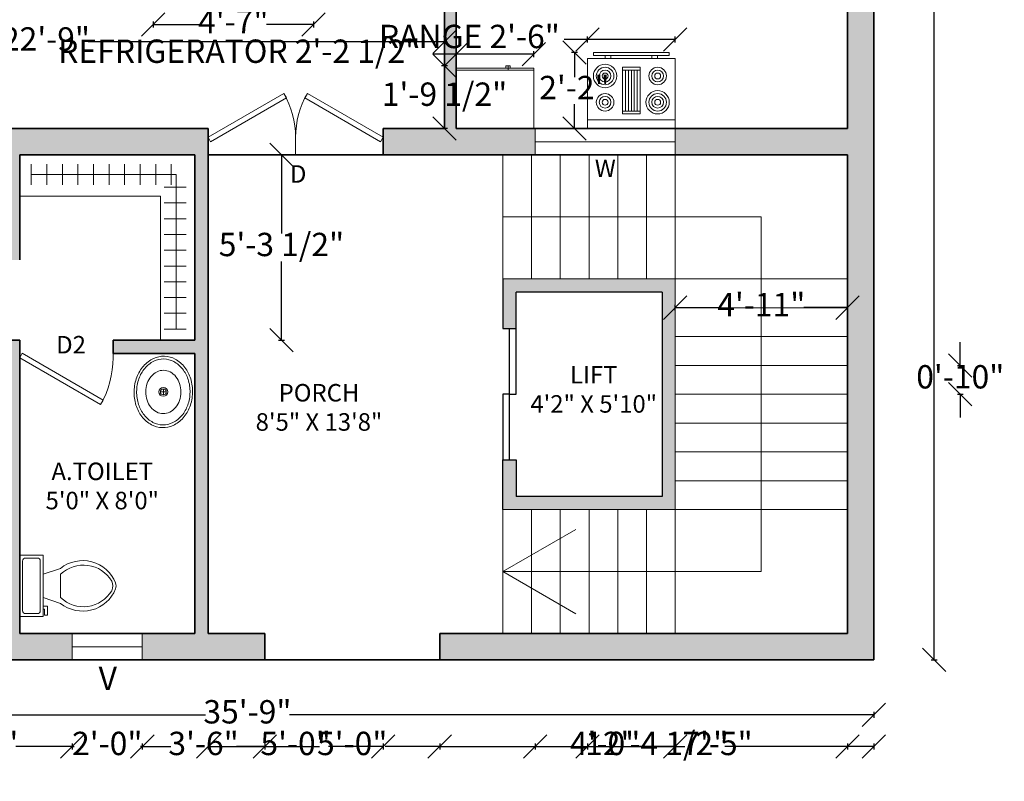
# Model space of a CAD drawing. Units: inches. Extents: x 2530 to 3100, y 543 to 1175.
# Tile 2 of 5: x 2762 to 3100, y 543 to 804. Entities that reach past the tile are written whole.
import ezdxf

# ---------------------------------------------------------------- set-up
doc = ezdxf.new("R2010")
doc.units = ezdxf.units.IN
for name, color, linetype, lineweight in [('A-ANNO-DIMS', 2, 'Continuous', 18), ('A-ANNO-TEXT', 7, 'Continuous', 18), ('A-AREA-IDEN', 7, 'Continuous', 18), ('A-DOOR', 3, 'Continuous', 18), ('A-EQPM', 8, 'Continuous', 18), ('A-FLOR-CASE', 172, 'Continuous', 13), ('A-FLOR-EVTR', 7, 'Continuous', 25), ('A-FLOR-FIXT', 8, 'Continuous', 18), ('A-FLOR-STRS', 7, 'Continuous', 18), ('A-GLAZ', 4, 'Continuous', 18), ('A-WALL', 7, 'Continuous', 35), ('A-WALL-PATT', 30, 'Continuous', 13)]:
    doc.layers.add(name, color=color, linetype=linetype, lineweight=lineweight)
doc.styles.get("Standard").update_dxf_attribs({"font": 'arial.ttf'})
doc.dimstyles.new('ISO-25', dxfattribs={"dimtxt": 8, "dimasz": 8, "dimexe": 1, "dimexo": 1, "dimtad": 0, "dimtih": 1, "dimtoh": 1, "dimlunit": 3, "dimtxsty": 'Standard', "dimblk": 'OBLIQUE', "dimcen": 2.5, "dimadec": 0, "dimazin": 0, "dimtfac": 1, "dimtmove": 0, "dimatfit": 3, "dimfxl": 1, "dimfxlon": 1, "dimarcsym": 0})

# ---------------------------------------------------------------- blocks, each defined once
blk = doc.blocks.new('*U10')
for p, q in [((0, 0), (0, 6)), ((32, 0), (32, 6))]:
    blk.add_line(p, q)
blk.add_lwpolyline([(0, 0), (27.71, -16), (28.59, -14.48), (0.87, 1.52)], close=True)
blk.add_arc((0, 0), 32, 330, 0)
blk = doc.blocks.new('*U9')
for p, q in [((0, 0), (0, -6)), ((30, 0), (30, -6))]:
    blk.add_line(p, q)
blk.add_lwpolyline([(0, 0), (25.98, 15), (26.86, 13.48), (0.87, -1.52)], close=True)
blk.add_arc((0, 0), 30, 0, 30)
blk = doc.blocks.new('*U8')
for p, q in [((-30, 0), (-30, -6)), ((0, 0), (0, -6))]:
    blk.add_line(p, q)
blk.add_lwpolyline([(0, 0), (-25.98, 15), (-26.86, 13.48), (-0.88, -1.52)], close=True)
blk.add_arc((0, 0), 30, 150, 180)
blk = doc.blocks.new('_Oblique')
at = {"color": 0, "linetype": 'ByBlock', "lineweight": -2}
blk.add_line((-0.5, -0.5), (0.5, 0.5), dxfattribs=at)
blk = doc.blocks.new('*D11')
at = {"layer": 'A-ANNO-DIMS', "color": 0, "lineweight": -2, "transparency": 16777216}
for p, q in [((2625.92, 566.6), (2625.92, 564.6)), ((3054.92, 566.6), (3054.92, 564.6)), ((2625.92, 565.6), (2826.05, 565.6)), ((3054.92, 565.6), (2854.78, 565.6))]:
    blk.add_line(p, q, dxfattribs=at)
at = {"layer": 'Defpoints', "color": 0, "transparency": 16777216}
for p in [(2625.92, 584.41), (3054.92, 584.41), (2625.92, 565.6)]:
    blk.add_point(p, dxfattribs=at)
at = {"layer": 'A-ANNO-DIMS', "color": 0, "lineweight": -2, "transparency": 16777216, "xscale": 8, "yscale": 8, "zscale": 8, "rotation": 180}
blk.add_blockref('_Oblique', (2625.92, 565.6), dxfattribs=at)
at = {"layer": 'A-ANNO-DIMS', "color": 0, "lineweight": -2, "transparency": 16777216, "xscale": 8, "yscale": 8, "zscale": 8}
blk.add_blockref('_Oblique', (3054.92, 565.6), dxfattribs=at)
at = {"layer": 'A-ANNO-DIMS', "color": 0, "transparency": 16777216, "insert": (2840.42, 565.6), "char_height": 8, "attachment_point": 5}
blk.add_mtext('35\'-9"', dxfattribs=at)
blk = doc.blocks.new('*D12')
at = {"layer": 'A-ANNO-DIMS', "color": 0, "lineweight": -2, "transparency": 16777216}
for p, q in [((3074.63, 1133.41), (3076.63, 1133.41)), ((3075.63, 1133.41), (3075.63, 863.62)), ((3075.63, 584.41), (3075.63, 854.2)), ((3074.63, 584.41), (3076.63, 584.41))]:
    blk.add_line(p, q, dxfattribs=at)
at = {"layer": 'Defpoints', "color": 0, "transparency": 16777216}
for p in [(3054.92, 1133.41), (3054.92, 584.41), (3075.63, 584.41)]:
    blk.add_point(p, dxfattribs=at)
at = {"layer": 'A-ANNO-DIMS', "color": 0, "lineweight": -2, "transparency": 16777216, "xscale": 8, "yscale": 8, "zscale": 8}
for p, rotation in [((3075.63, 1133.41), 90), ((3075.63, 584.41), 270)]:
    blk.add_blockref('_Oblique', p, dxfattribs=dict(at, rotation=rotation))
at = {"layer": 'A-ANNO-DIMS', "color": 0, "transparency": 16777216, "insert": (3075.63, 858.91), "char_height": 8, "attachment_point": 5}
blk.add_mtext('45\'-9"', dxfattribs=at)
blk = doc.blocks.new('Range-Oven - 30 in top')
for p, q in [((0, -3), (30, -3)), ((12, -6), (18, -6)), ((13, -20), (13, -6)), ((14, -6), (14, -20)), ((15, -20), (15, -6)), ((16, -6), (16, -20)), ((17, -20), (17, -6)), ((18, -20), (12, -20)), ((6, -24), (6, -25)), ((8, -25), (8, -24)), ((22, -25), (22, -24)), ((24, -24), (24, -25))]:
    blk.add_line(p, q)
for points in [[(0, -24), (0, 0), (30, 0), (30, -24)], [(12, -21), (12, -5), (18, -5), (18, -21)], [(2, -26), (2, -25), (28, -25), (28, -26)]]:
    blk.add_lwpolyline(points, close=True)
for centre, radius in [((6, -9), 4), ((6, -9), 3), ((24, -9), 3), ((6, -9), 2), ((6, -9), 1), ((24, -9), 2), ((24, -9), 1), ((6, -18), 3), ((6, -18), 2), ((24, -18), 4), ((24, -18), 3), ((24, -18), 2), ((6, -18), 1), ((24, -18), 1)]:
    blk.add_circle(centre, radius)
blk = doc.blocks.new('Refrigerator-2 door - 36 in top')
for p, q in [((0, -26.999999), (36, -26.999999)), ((12, -26.999999), (12, -28.999999)), ((11, -27.999999), (11, -28.999999)), ((11, -28.999999), (13, -28.999999)), ((13, -28.999999), (13, -27.999999))]:
    blk.add_line(p, q)
blk.add_lwpolyline([(0, -27.999999), (0, 0), (36, 0), (36, -27.999999)], close=True)
blk = doc.blocks.new('Toilet - top')
for p, q in [((9.5, -6), (9.5, -2)), ((-10, -8.5), (-8, -8.5)), ((-10, -9.5), (-10, -8.5)), ((-7, -9.5), (-10, -9.5)), ((-8, -8.5), (-8, -8)), ((-7, -8), (-7, -9.5)), ((-4, -8), (-6, -14)), ((4, -8), (6, -14)), ((4, -14), (-4, -14))]:
    blk.add_line(p, q)
blk.add_lwpolyline([(10.5, -8), (10.5, 0), (-10.5, 0), (-10.5, -8)], close=True)
for points in [[(-9.5, -2), (-9.5, -6)], [(8.5, -1), (-8.5, -1)], [(-8.5, -7), (8.5, -7)]]:
    blk.add_lwpolyline(points)
for centre, radius, start, end in [((-8.62, -1.88), 0.884, 81.8699, 188.1301), ((8.62, -1.88), 0.884, 351.8699, 98.1301), ((-8.62, -6.12), 0.884, 171.8699, 278.1301), ((8.62, -6.12), 0.884, 261.8699, 8.1301), ((3.52, -21.58), 12.17, 141.4691, 247.9714), ((4.2, -21.82), 11.33, 136.3677, 238.9468), ((-3.52, -21.58), 12.17, 292.0284, 38.5307), ((-4.2, -21.82), 11.33, 301.053, 43.6321), ((0, -27.88), 4, 245.7318, 294.2682), ((0, -29), 4, 254.8605, 285.1395)]:
    blk.add_arc(centre, radius, start, end)
blk = doc.blocks.new('Sink - Oval top')
for p, q in [((-1, 0), (1, 0)), ((0, 1), (0, -1))]:
    blk.add_line(p, q)
for points in [[(-12.23, 0.39, 0.117634), (-11.46, -3.36, 0.104469), (-8.88, -6.8, 0.090016), (-5.08, -9.07, 0.08192), (-0.32, -10.02, 0.08192), (4.49, -9.38, 0.090016), (8.42, -7.36, 0.104469), (11.22, -4.09, 0.117634), (12.23, -0.39, 0.117634), (11.46, 3.36, 0.104469), (8.88, 6.8, 0.090016), (5.08, 9.07, 0.08192), (0.32, 10.02, 0.08192), (-4.49, 9.38, 0.090016), (-8.42, 7.36, 0.104469), (-11.22, 4.09, 0.117634)], [(-11.29, 0.16, 0.118622), (-10.52, -3.25, 0.104678), (-8.07, -6.36, 0.089562), (-4.54, -8.37, 0.081185), (-0.13, -9.15, 0.081185), (4.3, -8.49, 0.089562), (7.89, -6.58, 0.104678), (10.42, -3.55, 0.118622), (11.29, -0.16, 0.118622), (10.52, 3.25, 0.104678), (8.07, 6.36, 0.089562), (4.54, 8.37, 0.081185), (0.13, 9.15, 0.081185), (-4.3, 8.49, 0.089562), (-7.89, 6.58, 0.104678), (-10.42, 3.55, 0.118622)], [(-7.42, 0.08, 0.118283), (-6.91, -2.17, 0.104607), (-5.29, -4.21, 0.089718), (-2.97, -5.53, 0.081436), (-0.07, -6.04, 0.081436), (2.84, -5.59, 0.089718), (5.2, -4.33, 0.104607), (6.86, -2.32, 0.118283), (7.42, -0.08, 0.118283), (6.91, 2.17, 0.104607), (5.29, 4.21, 0.089718), (2.97, 5.53, 0.081436), (0.07, 6.04, 0.081436), (-2.84, 5.59, 0.089718), (-5.2, 4.33, 0.104607), (-6.86, 2.32, 0.118283)]]:
    blk.add_lwpolyline(points, format="xyb", close=True)
for radius in [1.5, 1]:
    blk.add_circle((0, 0), radius)
blk = doc.blocks.new('*D36')
at = {"layer": 'A-ANNO-DIMS', "color": 0, "lineweight": -2, "transparency": 16777216}
for p, q in [((2956.92, 796.91), (2948.92, 796.91)), ((2956.92, 795.91), (2956.92, 797.91)), ((2986.92, 796.91), (2956.92, 796.91)), ((2986.92, 795.91), (2986.92, 797.91))]:
    blk.add_line(p, q, dxfattribs=at)
at = {"layer": 'Defpoints', "color": 0, "transparency": 16777216}
for p in [(2956.92, 796.91), (2956.92, 792.41), (2986.92, 792.41)]:
    blk.add_point(p, dxfattribs=at)
at = {"layer": 'A-ANNO-DIMS', "color": 0, "lineweight": -2, "transparency": 16777216, "xscale": 8, "yscale": 8, "zscale": 8, "rotation": 180}
blk.add_blockref('_Oblique', (2956.92, 796.91), dxfattribs=at)
at = {"layer": 'A-ANNO-DIMS', "color": 0, "lineweight": -2, "transparency": 16777216, "xscale": 8, "yscale": 8, "zscale": 8}
blk.add_blockref('_Oblique', (2986.92, 796.91), dxfattribs=at)
at = {"layer": 'A-ANNO-DIMS', "color": 0, "transparency": 16777216, "insert": (2916.44, 796.91), "char_height": 8, "attachment_point": 5}
blk.add_mtext('RANGE 2\'-6"', dxfattribs=at)
blk = doc.blocks.new('*D37')
at = {"layer": 'A-ANNO-DIMS', "color": 0, "lineweight": -2, "transparency": 16777216}
for p, q in [((2953.42, 792.41), (2951.42, 792.41)), ((2952.42, 792.41), (2952.42, 784.05)), ((2952.42, 766.41), (2952.42, 774.77)), ((2953.42, 766.41), (2951.42, 766.41))]:
    blk.add_line(p, q, dxfattribs=at)
at = {"layer": 'Defpoints', "color": 0, "transparency": 16777216}
for p in [(2956.92, 792.41), (2952.42, 766.41), (2956.92, 766.41)]:
    blk.add_point(p, dxfattribs=at)
at = {"layer": 'A-ANNO-DIMS', "color": 0, "lineweight": -2, "transparency": 16777216, "xscale": 8, "yscale": 8, "zscale": 8}
for p, rotation in [((2952.42, 792.41), 90), ((2952.42, 766.41), 270)]:
    blk.add_blockref('_Oblique', p, dxfattribs=dict(at, rotation=rotation))
at = {"layer": 'A-ANNO-DIMS', "color": 0, "transparency": 16777216, "insert": (2952.42, 779.41), "char_height": 8, "attachment_point": 5}
blk.add_mtext('2\'-2"', dxfattribs=at)
blk = doc.blocks.new('*D38')
at = {"layer": 'A-ANNO-DIMS', "color": 0, "lineweight": -2, "transparency": 16777216}
for p, q in [((2911.92, 790.86), (2911.92, 792.86)), ((2938.56, 790.86), (2938.56, 792.86)), ((2911.92, 791.86), (2903.92, 791.86)), ((2938.56, 791.86), (2911.92, 791.86))]:
    blk.add_line(p, q, dxfattribs=at)
at = {"layer": 'Defpoints', "color": 0, "transparency": 16777216}
for p in [(2911.92, 791.86), (2911.92, 787.87), (2938.56, 787.87)]:
    blk.add_point(p, dxfattribs=at)
at = {"layer": 'A-ANNO-DIMS', "color": 0, "lineweight": -2, "transparency": 16777216, "xscale": 8, "yscale": 8, "zscale": 8, "rotation": 180}
blk.add_blockref('_Oblique', (2911.92, 791.86), dxfattribs=at)
at = {"layer": 'A-ANNO-DIMS', "color": 0, "lineweight": -2, "transparency": 16777216, "xscale": 8, "yscale": 8, "zscale": 8}
blk.add_blockref('_Oblique', (2938.56, 791.86), dxfattribs=at)
at = {"layer": 'A-ANNO-DIMS', "color": 0, "transparency": 16777216, "insert": (2837.6, 791.86), "char_height": 8, "attachment_point": 5}
blk.add_mtext('REFRIGERATOR 2\'-2 1/2"', dxfattribs=at)
blk = doc.blocks.new('*D39')
at = {"layer": 'A-ANNO-DIMS', "color": 0, "lineweight": -2, "transparency": 16777216}
for p, q in [((2908.92, 787.87), (2906.92, 787.87)), ((2907.92, 787.87), (2907.92, 781.9)), ((2907.92, 766.41), (2907.92, 772.38)), ((2908.92, 766.41), (2906.92, 766.41))]:
    blk.add_line(p, q, dxfattribs=at)
at = {"layer": 'Defpoints', "color": 0, "transparency": 16777216}
for p in [(2911.92, 787.87), (2907.92, 766.41), (2911.92, 766.41)]:
    blk.add_point(p, dxfattribs=at)
at = {"layer": 'A-ANNO-DIMS', "color": 0, "lineweight": -2, "transparency": 16777216, "xscale": 8, "yscale": 8, "zscale": 8}
for p, rotation in [((2907.92, 787.87), 90), ((2907.92, 766.41), 270)]:
    blk.add_blockref('_Oblique', p, dxfattribs=dict(at, rotation=rotation))
at = {"layer": 'A-ANNO-DIMS', "color": 0, "transparency": 16777216, "insert": (2907.92, 777.14), "char_height": 8, "attachment_point": 5}
blk.add_mtext('1\'-9 1/2"', dxfattribs=at)
blk = doc.blocks.new('*D43')
at = {"layer": 'A-ANNO-DIMS', "color": 0, "lineweight": -2, "transparency": 16777216}
for p, q in [((2808.08, 803.02), (2808.08, 801.02)), ((2863.08, 803.02), (2863.08, 801.02)), ((2808.08, 802.02), (2824.16, 802.02)), ((2863.08, 802.02), (2847, 802.02))]:
    blk.add_line(p, q, dxfattribs=at)
at = {"layer": 'Defpoints', "color": 0, "transparency": 16777216}
for p in [(2808.08, 815.67), (2863.08, 815.67), (2863.08, 802.02)]:
    blk.add_point(p, dxfattribs=at)
at = {"layer": 'A-ANNO-DIMS', "color": 0, "lineweight": -2, "transparency": 16777216, "xscale": 8, "yscale": 8, "zscale": 8, "rotation": 180}
blk.add_blockref('_Oblique', (2808.08, 802.02), dxfattribs=at)
at = {"layer": 'A-ANNO-DIMS', "color": 0, "lineweight": -2, "transparency": 16777216, "xscale": 8, "yscale": 8, "zscale": 8}
blk.add_blockref('_Oblique', (2863.08, 802.02), dxfattribs=at)
at = {"layer": 'A-ANNO-DIMS', "color": 0, "transparency": 16777216, "insert": (2835.58, 802.02), "char_height": 8, "attachment_point": 5}
blk.add_mtext('4\'-7"', dxfattribs=at)
blk = doc.blocks.new('*D46')
at = {"layer": 'A-ANNO-DIMS', "color": 0, "lineweight": -2, "transparency": 16777216}
for p, q in [((2634.92, 795.06), (2634.92, 797.06)), ((2634.92, 796.06), (2756.98, 796.06)), ((2907.92, 796.06), (2785.85, 796.06)), ((2907.92, 795.06), (2907.92, 797.06))]:
    blk.add_line(p, q, dxfattribs=at)
at = {"layer": 'Defpoints', "color": 0, "transparency": 16777216}
for p in [(2907.92, 796.06), (2634.92, 766.41), (2907.92, 766.41)]:
    blk.add_point(p, dxfattribs=at)
at = {"layer": 'A-ANNO-DIMS', "color": 0, "lineweight": -2, "transparency": 16777216, "xscale": 8, "yscale": 8, "zscale": 8, "rotation": 180}
blk.add_blockref('_Oblique', (2634.92, 796.06), dxfattribs=at)
at = {"layer": 'A-ANNO-DIMS', "color": 0, "lineweight": -2, "transparency": 16777216, "xscale": 8, "yscale": 8, "zscale": 8}
blk.add_blockref('_Oblique', (2907.92, 796.06), dxfattribs=at)
at = {"layer": 'A-ANNO-DIMS', "color": 0, "transparency": 16777216, "insert": (2771.42, 796.06), "char_height": 8, "attachment_point": 5}
blk.add_mtext('22\'-9"', dxfattribs=at)
blk = doc.blocks.new('*D49')
at = {"layer": 'A-ANNO-DIMS', "color": 0, "lineweight": -2, "transparency": 16777216}
for p, q in [((2826.92, 555.76), (2826.92, 553.76)), ((2826.92, 554.76), (2845.66, 554.76)), ((2886.92, 554.76), (2868.18, 554.76)), ((2886.92, 555.76), (2886.92, 553.76))]:
    blk.add_line(p, q, dxfattribs=at)
at = {"layer": 'Defpoints', "color": 0, "transparency": 16777216}
for p in [(2826.92, 757.41), (2886.92, 757.41), (2886.92, 554.76)]:
    blk.add_point(p, dxfattribs=at)
at = {"layer": 'A-ANNO-DIMS', "color": 0, "lineweight": -2, "transparency": 16777216, "xscale": 8, "yscale": 8, "zscale": 8, "rotation": 180}
blk.add_blockref('_Oblique', (2826.92, 554.76), dxfattribs=at)
at = {"layer": 'A-ANNO-DIMS', "color": 0, "lineweight": -2, "transparency": 16777216, "xscale": 8, "yscale": 8, "zscale": 8}
blk.add_blockref('_Oblique', (2886.92, 554.76), dxfattribs=at)
at = {"layer": 'A-ANNO-DIMS', "color": 0, "transparency": 16777216, "insert": (2856.92, 554.76), "char_height": 8, "attachment_point": 5}
blk.add_mtext('5\'-0"', dxfattribs=at)
blk = doc.blocks.new('*D58')
at = {"layer": 'A-ANNO-DIMS', "color": 0, "lineweight": -2, "transparency": 16777216}
for p, q in [((2719.35, 555.76), (2719.35, 553.76)), ((2719.35, 554.76), (2738.63, 554.76)), ((2780.42, 554.76), (2761.14, 554.76)), ((2780.42, 555.76), (2780.42, 553.76))]:
    blk.add_line(p, q, dxfattribs=at)
at = {"layer": 'Defpoints', "color": 0, "transparency": 16777216}
for p in [(2719.35, 584.41), (2780.42, 584.41), (2780.42, 554.76)]:
    blk.add_point(p, dxfattribs=at)
at = {"layer": 'A-ANNO-DIMS', "color": 0, "lineweight": -2, "transparency": 16777216, "xscale": 8, "yscale": 8, "zscale": 8, "rotation": 180}
blk.add_blockref('_Oblique', (2719.35, 554.76), dxfattribs=at)
at = {"layer": 'A-ANNO-DIMS', "color": 0, "lineweight": -2, "transparency": 16777216, "xscale": 8, "yscale": 8, "zscale": 8}
blk.add_blockref('_Oblique', (2780.42, 554.76), dxfattribs=at)
at = {"layer": 'A-ANNO-DIMS', "color": 0, "transparency": 16777216, "insert": (2749.88, 554.76), "char_height": 8, "attachment_point": 5}
blk.add_mtext('5\'-1"', dxfattribs=at)
blk = doc.blocks.new('*D59')
at = {"layer": 'A-ANNO-DIMS', "color": 0, "lineweight": -2, "transparency": 16777216}
for p, q in [((2780.42, 555.76), (2780.42, 553.76)), ((2780.42, 554.76), (2781.09, 554.76)), ((2804.42, 554.76), (2803.74, 554.76)), ((2804.42, 555.76), (2804.42, 553.76))]:
    blk.add_line(p, q, dxfattribs=at)
at = {"layer": 'Defpoints', "color": 0, "transparency": 16777216}
for p in [(2780.42, 584.41), (2804.42, 584.41), (2804.42, 554.76)]:
    blk.add_point(p, dxfattribs=at)
at = {"layer": 'A-ANNO-DIMS', "color": 0, "lineweight": -2, "transparency": 16777216, "xscale": 8, "yscale": 8, "zscale": 8, "rotation": 180}
blk.add_blockref('_Oblique', (2780.42, 554.76), dxfattribs=at)
at = {"layer": 'A-ANNO-DIMS', "color": 0, "lineweight": -2, "transparency": 16777216, "xscale": 8, "yscale": 8, "zscale": 8}
blk.add_blockref('_Oblique', (2804.42, 554.76), dxfattribs=at)
at = {"layer": 'A-ANNO-DIMS', "color": 0, "transparency": 16777216, "insert": (2792.42, 554.76), "char_height": 8, "attachment_point": 5}
blk.add_mtext('2\'-0"', dxfattribs=at)
blk = doc.blocks.new('*D60')
at = {"layer": 'A-ANNO-DIMS', "color": 0, "lineweight": -2, "transparency": 16777216}
for p, q in [((2804.42, 555.76), (2804.42, 553.76)), ((2804.42, 554.76), (2814.13, 554.76)), ((2846.36, 554.76), (2836.64, 554.76)), ((2846.36, 555.76), (2846.36, 553.76))]:
    blk.add_line(p, q, dxfattribs=at)
at = {"layer": 'Defpoints', "color": 0, "transparency": 16777216}
for p in [(2804.42, 584.41), (2846.36, 584.41), (2846.36, 554.76)]:
    blk.add_point(p, dxfattribs=at)
at = {"layer": 'A-ANNO-DIMS', "color": 0, "lineweight": -2, "transparency": 16777216, "xscale": 8, "yscale": 8, "zscale": 8, "rotation": 180}
blk.add_blockref('_Oblique', (2804.42, 554.76), dxfattribs=at)
at = {"layer": 'A-ANNO-DIMS', "color": 0, "lineweight": -2, "transparency": 16777216, "xscale": 8, "yscale": 8, "zscale": 8}
blk.add_blockref('_Oblique', (2846.36, 554.76), dxfattribs=at)
at = {"layer": 'A-ANNO-DIMS', "color": 0, "transparency": 16777216, "insert": (2825.39, 554.76), "char_height": 8, "attachment_point": 5}
blk.add_mtext('3\'-6"', dxfattribs=at)
blk = doc.blocks.new('*D61')
at = {"layer": 'A-ANNO-DIMS', "color": 0, "lineweight": -2, "transparency": 16777216}
for p, q in [((2846.36, 555.76), (2846.36, 553.76)), ((2846.36, 554.76), (2865.05, 554.76)), ((2906.26, 554.76), (2887.57, 554.76)), ((2906.26, 555.76), (2906.26, 553.76))]:
    blk.add_line(p, q, dxfattribs=at)
at = {"layer": 'Defpoints', "color": 0, "transparency": 16777216}
for p in [(2846.36, 584.41), (2906.26, 584.41), (2906.26, 554.76)]:
    blk.add_point(p, dxfattribs=at)
at = {"layer": 'A-ANNO-DIMS', "color": 0, "lineweight": -2, "transparency": 16777216, "xscale": 8, "yscale": 8, "zscale": 8, "rotation": 180}
blk.add_blockref('_Oblique', (2846.36, 554.76), dxfattribs=at)
at = {"layer": 'A-ANNO-DIMS', "color": 0, "lineweight": -2, "transparency": 16777216, "xscale": 8, "yscale": 8, "zscale": 8}
blk.add_blockref('_Oblique', (2906.26, 554.76), dxfattribs=at)
at = {"layer": 'A-ANNO-DIMS', "color": 0, "transparency": 16777216, "insert": (2876.31, 554.76), "char_height": 8, "attachment_point": 5}
blk.add_mtext('5\'-0"', dxfattribs=at)
blk = doc.blocks.new('*D66')
at = {"layer": 'A-ANNO-DIMS', "color": 0, "lineweight": -2, "transparency": 16777216}
for p, q in [((2938.92, 555.76), (2938.92, 553.76)), ((2938.92, 554.76), (2951.5, 554.76)), ((2986.92, 554.76), (2974.34, 554.76)), ((2986.92, 555.76), (2986.92, 553.76))]:
    blk.add_line(p, q, dxfattribs=at)
at = {"layer": 'Defpoints', "color": 0, "transparency": 16777216}
for p in [(2938.92, 757.41), (2986.92, 757.41), (2986.92, 554.76)]:
    blk.add_point(p, dxfattribs=at)
at = {"layer": 'A-ANNO-DIMS', "color": 0, "lineweight": -2, "transparency": 16777216, "xscale": 8, "yscale": 8, "zscale": 8, "rotation": 180}
blk.add_blockref('_Oblique', (2938.92, 554.76), dxfattribs=at)
at = {"layer": 'A-ANNO-DIMS', "color": 0, "lineweight": -2, "transparency": 16777216, "xscale": 8, "yscale": 8, "zscale": 8}
blk.add_blockref('_Oblique', (2986.92, 554.76), dxfattribs=at)
at = {"layer": 'A-ANNO-DIMS', "color": 0, "transparency": 16777216, "insert": (2962.92, 554.76), "char_height": 8, "attachment_point": 5}
blk.add_mtext('4\'-0"', dxfattribs=at)
blk = doc.blocks.new('*D67')
at = {"layer": 'A-ANNO-DIMS', "color": 0, "lineweight": -2, "transparency": 16777216}
for p, q in [((2986.92, 704.06), (2986.92, 706.06)), ((2986.92, 705.06), (3001.89, 705.06)), ((3045.92, 705.06), (3030.94, 705.06)), ((3045.92, 704.06), (3045.92, 706.06))]:
    blk.add_line(p, q, dxfattribs=at)
at = {"layer": 'Defpoints', "color": 0, "transparency": 16777216}
for p in [(3045.92, 705.06), (2986.92, 675.41), (3045.92, 675.41)]:
    blk.add_point(p, dxfattribs=at)
at = {"layer": 'A-ANNO-DIMS', "color": 0, "lineweight": -2, "transparency": 16777216, "xscale": 8, "yscale": 8, "zscale": 8, "rotation": 180}
blk.add_blockref('_Oblique', (2986.92, 705.06), dxfattribs=at)
at = {"layer": 'A-ANNO-DIMS', "color": 0, "lineweight": -2, "transparency": 16777216, "xscale": 8, "yscale": 8, "zscale": 8}
blk.add_blockref('_Oblique', (3045.92, 705.06), dxfattribs=at)
at = {"layer": 'A-ANNO-DIMS', "color": 0, "transparency": 16777216, "insert": (3016.42, 705.06), "char_height": 8, "attachment_point": 5}
blk.add_mtext('4\'-11"', dxfattribs=at)
blk = doc.blocks.new('*D68')
at = {"layer": 'A-ANNO-DIMS', "color": 0, "lineweight": -2, "transparency": 16777216}
for p, q in [((2597.27, 635.91), (2595.27, 635.91)), ((2596.27, 635.91), (2596.27, 619.42)), ((2596.27, 593.41), (2596.27, 609.89)), ((2597.27, 593.41), (2595.27, 593.41))]:
    blk.add_line(p, q, dxfattribs=at)
at = {"layer": 'Defpoints', "color": 0, "transparency": 16777216}
for p in [(2596.27, 635.91), (2927.92, 635.91), (2927.92, 593.41)]:
    blk.add_point(p, dxfattribs=at)
at = {"layer": 'A-ANNO-DIMS', "color": 0, "lineweight": -2, "transparency": 16777216, "xscale": 8, "yscale": 8, "zscale": 8}
for p, rotation in [((2596.27, 635.91), 90), ((2596.27, 593.41), 270)]:
    blk.add_blockref('_Oblique', p, dxfattribs=dict(at, rotation=rotation))
at = {"layer": 'A-ANNO-DIMS', "color": 0, "transparency": 16777216, "insert": (2596.27, 614.66), "char_height": 8, "attachment_point": 5}
blk.add_mtext('3\'-6 1/2"', dxfattribs=at)
blk = doc.blocks.new('*D69')
at = {"layer": 'A-ANNO-DIMS', "color": 0, "lineweight": -2, "transparency": 16777216}
for p, q in [((2956.92, 555.76), (2956.92, 553.76)), ((2956.92, 554.76), (2990.19, 554.76)), ((3045.92, 554.76), (3012.64, 554.76)), ((3045.92, 555.76), (3045.92, 553.76))]:
    blk.add_line(p, q, dxfattribs=at)
at = {"layer": 'Defpoints', "color": 0, "transparency": 16777216}
for p in [(2956.92, 944.41), (3045.92, 944.41), (3045.92, 554.76)]:
    blk.add_point(p, dxfattribs=at)
at = {"layer": 'A-ANNO-DIMS', "color": 0, "lineweight": -2, "transparency": 16777216, "xscale": 8, "yscale": 8, "zscale": 8, "rotation": 180}
blk.add_blockref('_Oblique', (2956.92, 554.76), dxfattribs=at)
at = {"layer": 'A-ANNO-DIMS', "color": 0, "lineweight": -2, "transparency": 16777216, "xscale": 8, "yscale": 8, "zscale": 8}
blk.add_blockref('_Oblique', (3045.92, 554.76), dxfattribs=at)
at = {"layer": 'A-ANNO-DIMS', "color": 0, "transparency": 16777216, "insert": (3001.42, 554.76), "char_height": 8, "attachment_point": 5}
blk.add_mtext('7\'-5"', dxfattribs=at)
blk = doc.blocks.new('*D72')
at = {"layer": 'A-ANNO-DIMS', "color": 0, "lineweight": -2, "transparency": 16777216}
for p, q in [((2906.26, 555.76), (2906.26, 553.76)), ((2906.26, 554.76), (2957.28, 554.76)), ((3054.92, 554.76), (3003.9, 554.76)), ((3054.92, 555.76), (3054.92, 553.76))]:
    blk.add_line(p, q, dxfattribs=at)
at = {"layer": 'Defpoints', "color": 0, "transparency": 16777216}
for p in [(2906.26, 584.41), (3054.92, 584.41), (3054.92, 554.76)]:
    blk.add_point(p, dxfattribs=at)
at = {"layer": 'A-ANNO-DIMS', "color": 0, "lineweight": -2, "transparency": 16777216, "xscale": 8, "yscale": 8, "zscale": 8, "rotation": 180}
blk.add_blockref('_Oblique', (2906.26, 554.76), dxfattribs=at)
at = {"layer": 'A-ANNO-DIMS', "color": 0, "lineweight": -2, "transparency": 16777216, "xscale": 8, "yscale": 8, "zscale": 8}
blk.add_blockref('_Oblique', (3054.92, 554.76), dxfattribs=at)
at = {"layer": 'A-ANNO-DIMS', "color": 0, "transparency": 16777216, "insert": (2980.59, 554.76), "char_height": 8, "attachment_point": 5}
blk.add_mtext('12\'-4 1/2"', dxfattribs=at)
blk = doc.blocks.new('*D74')
at = {"layer": 'A-ANNO-DIMS', "color": 0, "lineweight": -2, "transparency": 16777216}
for p, q in [((3084.57, 685.28), (3084.57, 693.28)), ((3083.57, 685.28), (3085.57, 685.28)), ((3084.57, 685.28), (3084.57, 685.05)), ((3083.57, 675.41), (3085.57, 675.41)), ((3084.57, 675.41), (3084.57, 675.64)), ((3084.57, 675.41), (3084.57, 667.41))]:
    blk.add_line(p, q, dxfattribs=at)
at = {"layer": 'Defpoints', "color": 0, "transparency": 16777216}
for p in [(3045.92, 685.28), (3084.57, 685.28), (3045.92, 675.41)]:
    blk.add_point(p, dxfattribs=at)
at = {"layer": 'A-ANNO-DIMS', "color": 0, "lineweight": -2, "transparency": 16777216, "xscale": 8, "yscale": 8, "zscale": 8}
for p, rotation in [((3084.57, 685.28), 270), ((3084.57, 675.41), 90)]:
    blk.add_blockref('_Oblique', p, dxfattribs=dict(at, rotation=rotation))
at = {"layer": 'A-ANNO-DIMS', "color": 0, "transparency": 16777216, "insert": (3084.57, 680.34), "char_height": 8, "attachment_point": 5}
blk.add_mtext('0\'-10"', dxfattribs=at)
blk = doc.blocks.new('*D77')
at = {"layer": 'A-ANNO-DIMS', "color": 0, "lineweight": -2, "transparency": 16777216}
for p, q in [((2938.56, 1162.06), (2938.56, 1164.06)), ((2956.92, 1162.06), (2956.92, 1164.06)), ((2938.56, 1163.06), (2956.92, 1163.06)), ((2956.92, 1163.06), (2964.92, 1163.06))]:
    blk.add_line(p, q, dxfattribs=at)
at = {"layer": 'Defpoints', "color": 0, "transparency": 16777216}
for p in [(2956.92, 1163.06), (2956.92, 790.41), (2938.56, 787.13)]:
    blk.add_point(p, dxfattribs=at)
at = {"layer": 'A-ANNO-DIMS', "color": 0, "lineweight": -2, "transparency": 16777216, "xscale": 8, "yscale": 8, "zscale": 8, "rotation": 180}
blk.add_blockref('_Oblique', (2938.56, 1163.06), dxfattribs=at)
at = {"layer": 'A-ANNO-DIMS', "color": 0, "lineweight": -2, "transparency": 16777216, "xscale": 8, "yscale": 8, "zscale": 8}
blk.add_blockref('_Oblique', (2956.92, 1163.06), dxfattribs=at)
at = {"layer": 'A-ANNO-DIMS', "color": 0, "transparency": 16777216, "insert": (2985.12, 1163.06), "char_height": 8, "attachment_point": 5}
blk.add_mtext('1\'-6 1/2"', dxfattribs=at)
blk = doc.blocks.new('*D84')
at = {"layer": 'A-ANNO-DIMS', "color": 0, "lineweight": -2, "transparency": 16777216}
for p, q in [((2851.07, 757.41), (2853.07, 757.41)), ((2852.07, 757.41), (2852.07, 730.42)), ((2852.07, 693.91), (2852.07, 720.89)), ((2851.07, 693.91), (2853.07, 693.91))]:
    blk.add_line(p, q, dxfattribs=at)
at = {"layer": 'Defpoints', "color": 0, "transparency": 16777216}
for p in [(2822.42, 757.41), (2822.42, 693.91), (2852.07, 693.91)]:
    blk.add_point(p, dxfattribs=at)
at = {"layer": 'A-ANNO-DIMS', "color": 0, "lineweight": -2, "transparency": 16777216, "xscale": 8, "yscale": 8, "zscale": 8}
for p, rotation in [((2852.07, 757.41), 90), ((2852.07, 693.91), 270)]:
    blk.add_blockref('_Oblique', p, dxfattribs=dict(at, rotation=rotation))
at = {"layer": 'A-ANNO-DIMS', "color": 0, "transparency": 16777216, "insert": (2852.07, 725.66), "char_height": 8, "attachment_point": 5}
blk.add_mtext('5\'-3 1/2"', dxfattribs=at)

msp = doc.modelspace()

# ---------------------------------------------------------------- hatches: boundary and pattern name
at = {"layer": 'A-WALL-PATT'}
h = msp.add_hatch(color=256, dxfattribs=at)
h.dxf.hatch_style = 1
h.paths.add_polyline_path([(2676.945, 1133.407), (2625.918, 1133.407), (2625.918, 584.407), (2673.585, 584.407), (2673.585, 593.407), (2634.918, 593.407), (2634.918, 757.407), (2717.918, 757.407), (2717.918, 766.407), (2634.918, 766.407), (2634.918, 944.407), (2772.918, 944.407), (2772.918, 948.407), (2634.918, 948.407), (2634.918, 1124.407), (2676.945, 1124.407)])
h.paths.add_polyline_path([(2822.346, 1133.407), (2739.946, 1133.407), (2739.946, 1124.407), (2808.918, 1124.407), (2808.918, 1070.407), (2812.918, 1070.407), (2812.918, 1124.407), (2822.346, 1124.407)])
h.paths.add_polyline_path([(2939.91, 1133.407), (2855.561, 1133.407), (2855.561, 1124.407), (2867.918, 1124.407), (2867.918, 1038.407), (2808.918, 1038.407), (2808.918, 944.407), (2871.918, 944.407), (2871.918, 1002.407), (2867.918, 1002.407), (2867.918, 948.407), (2812.918, 948.407), (2812.918, 1034.407), (2871.918, 1034.407), (2871.918, 1124.407), (2939.91, 1124.407)])
h.paths.add_polyline_path([(3054.918, 1133.407), (2997.969, 1133.407), (2997.969, 1124.407), (3045.918, 1124.407), (3045.918, 948.407), (2907.918, 948.407), (2907.918, 928.407), (2911.918, 928.407), (2911.918, 944.407), (2952.418, 944.407), (2952.418, 872.407), (2911.918, 872.407), (2911.918, 888.407), (2907.918, 888.407), (2907.918, 861.407), (2911.918, 861.407), (2911.918, 867.407), (2956.918, 867.407), (2956.918, 944.407), (3045.918, 944.407), (3045.918, 872.407), (2988.918, 872.407), (2988.918, 867.407), (3045.918, 867.407), (3045.918, 766.407), (2986.918, 766.407), (2986.918, 757.407), (3045.918, 757.407), (3045.918, 593.407), (2906.263, 593.407), (2906.263, 584.407), (3054.918, 584.407)])
h.paths.add_polyline_path([(2780.418, 593.407), (2762.418, 593.407), (2762.418, 693.907), (2757.918, 693.907), (2757.918, 593.407), (2719.35, 593.407), (2719.35, 584.407), (2780.418, 584.407)])
h.paths.add_polyline_path([(2846.356, 593.407), (2826.918, 593.407), (2826.918, 757.407), (2826.918, 766.407), (2822.418, 766.407), (2822.418, 693.907), (2794.418, 693.907), (2794.418, 689.407), (2822.418, 689.407), (2822.418, 593.407), (2804.418, 593.407), (2804.418, 584.407), (2846.356, 584.407)])
h.paths.add_polyline_path([(2938.918, 766.407), (2911.918, 766.407), (2911.918, 829.407), (2907.918, 829.407), (2907.918, 766.407), (2886.918, 766.407), (2886.918, 757.407), (2938.918, 757.407)])
h.paths.add_polyline_path([(2822.418, 766.407), (2757.918, 766.407), (2757.918, 757.407), (2757.918, 721.407), (2762.418, 721.407), (2762.418, 757.407), (2822.418, 757.407)])
h = msp.add_hatch(color=256, dxfattribs=at)
h.dxf.hatch_style = 1
h.paths.add_polyline_path([(2986.918, 714.907), (2927.918, 714.907), (2927.918, 697.907), (2932.418, 697.907), (2932.418, 710.407), (2982.418, 710.407), (2982.418, 640.407), (2932.418, 640.407), (2932.418, 652.907), (2927.918, 652.907), (2927.918, 635.907), (2986.918, 635.907)])

# ---------------------------------------------------------------- linework, layer by layer
at = {"layer": 'A-FLOR-CASE'}
for p, q in [((2766.398, 754.222), (2766.398, 747.142)), ((2771.726, 754.221), (2771.726, 747.141)), ((2777.054, 754.221), (2777.054, 747.141)), ((2782.382, 754.22), (2782.382, 747.14)), ((2787.71, 754.219), (2787.71, 747.139)), ((2793.038, 754.219), (2793.038, 747.139)), ((2798.366, 754.218), (2798.366, 747.138)), ((2803.693, 754.218), (2803.693, 747.138)), ((2809.021, 754.217), (2809.021, 747.137)), ((2814.349, 754.217), (2814.349, 747.137)), ((2766.398, 750.677), (2815.993, 750.677)), ((2815.993, 750.677), (2815.993, 697.718)), ((2811.85, 746.306), (2819.41, 746.306)), ((2762.418, 743.237), (2810.697, 743.237)), ((2810.697, 743.237), (2810.697, 693.907)), ((2811.85, 740.907), (2819.41, 740.907)), ((2811.85, 735.508), (2819.41, 735.508)), ((2811.85, 730.11), (2819.41, 730.11)), ((2811.85, 724.711), (2819.41, 724.711)), ((2811.85, 719.313), (2819.41, 719.313)), ((2811.85, 713.914), (2819.41, 713.914)), ((2811.85, 708.515), (2819.41, 708.515)), ((2811.85, 703.117), (2819.41, 703.117)), ((2811.85, 697.718), (2819.41, 697.718))]:
    msp.add_line(p, q, dxfattribs=at)
at = {"layer": 'A-FLOR-EVTR'}
for p, q in [((2927.918, 714.907), (2927.918, 697.907)), ((2982.418, 710.407), (2932.418, 710.407)), ((2932.418, 697.907), (2932.418, 710.407)), ((2982.418, 710.407), (2982.418, 640.407)), ((2927.918, 697.907), (2932.418, 697.907)), ((2930.168, 652.907), (2930.168, 697.907)), ((2932.418, 675.407), (2932.418, 697.907)), ((2930.168, 675.407), (2927.918, 675.407)), ((2927.918, 675.407), (2927.918, 652.907)), ((2930.168, 675.407), (2932.418, 675.407)), ((2927.918, 635.907), (2927.918, 652.907)), ((2927.918, 652.907), (2932.418, 652.907)), ((2932.418, 652.907), (2932.418, 640.407)), ((2982.418, 640.407), (2932.418, 640.407))]:
    msp.add_line(p, q, dxfattribs=at)
at = {"layer": 'A-FLOR-STRS'}
for p, q in [((2927.918, 757.407), (2927.918, 714.907)), ((2937.751, 757.407), (2937.751, 714.907)), ((2947.584, 757.407), (2947.584, 714.907)), ((2957.418, 757.407), (2957.418, 714.907)), ((2967.251, 757.407), (2967.251, 714.907)), ((2977.084, 757.407), (2977.084, 714.907)), ((2986.918, 757.407), (2986.918, 593.407)), ((2927.918, 736.157), (3016.418, 736.157)), ((3016.418, 736.157), (3016.418, 614.657)), ((2986.918, 714.907), (2927.918, 714.907)), ((3045.918, 714.907), (2986.918, 714.907)), ((3045.918, 705.032), (2986.918, 705.032)), ((3045.918, 695.157), (2986.918, 695.157)), ((3045.918, 685.282), (2986.918, 685.282)), ((3045.918, 675.407), (2986.918, 675.407)), ((3045.918, 665.532), (2986.918, 665.532)), ((3045.918, 655.657), (2986.918, 655.657)), ((3045.918, 645.782), (2986.918, 645.782)), ((3045.918, 635.907), (2927.918, 635.907)), ((2927.918, 635.907), (2927.918, 593.407)), ((2937.748, 635.907), (2937.748, 593.407)), ((2947.578, 635.907), (2947.578, 593.407)), ((2957.408, 635.907), (2957.408, 593.407)), ((2967.238, 635.907), (2967.238, 593.407)), ((2977.068, 635.907), (2977.068, 593.407)), ((2927.918, 614.657), (2952.953, 629.111)), ((3016.418, 614.657), (2927.918, 614.657)), ((2927.918, 614.657), (2952.953, 600.203))]:
    msp.add_line(p, q, dxfattribs=at)
at = {"layer": 'A-GLAZ'}
for p, q in [((2938.918, 757.407), (2938.918, 766.407)), ((2986.918, 757.407), (2986.918, 766.407)), ((2938.918, 761.907), (2986.918, 761.907)), ((2780.418, 593.407), (2780.418, 584.407)), ((2804.418, 593.407), (2804.418, 584.407)), ((2804.418, 588.907), (2780.418, 588.907))]:
    msp.add_line(p, q, dxfattribs=at)
at = {"layer": 'A-WALL'}
for p, q in [((3054.918, 584.407), (3054.918, 1133.407)), ((3045.918, 766.407), (3045.918, 867.407)), ((2907.918, 766.407), (2907.918, 829.407)), ((2911.918, 766.407), (2911.918, 829.407)), ((2826.918, 766.407), (2757.918, 766.407)), ((2826.918, 757.407), (2826.918, 766.407)), ((2907.918, 766.407), (2886.918, 766.407)), ((2886.918, 757.407), (2886.918, 766.407)), ((3045.918, 766.407), (2911.918, 766.407)), ((2762.418, 757.407), (2762.418, 721.407)), ((2822.418, 757.407), (2762.418, 757.407)), ((2822.418, 757.407), (2822.418, 693.907)), ((2826.918, 757.407), (2826.918, 593.407)), ((3045.918, 757.407), (2826.918, 757.407)), ((3045.918, 593.407), (3045.918, 757.407)), ((2757.918, 693.907), (2762.418, 693.907)), ((2762.418, 693.907), (2762.418, 593.407)), ((2794.418, 689.407), (2794.418, 693.907)), ((2794.418, 693.907), (2822.418, 693.907)), ((2794.418, 689.407), (2822.418, 689.407)), ((2822.418, 689.407), (2822.418, 593.407)), ((2762.418, 593.407), (2822.418, 593.407)), ((2826.918, 593.407), (2846.356, 593.407)), ((2846.356, 593.407), (2846.356, 584.407)), ((2906.263, 593.407), (2906.263, 584.407)), ((2906.263, 593.407), (3045.918, 593.407)), ((2625.918, 584.407), (3054.918, 584.407))]:
    msp.add_line(p, q, dxfattribs=at)

# ---------------------------------------------------------------- block references
at = {"layer": 'A-DOOR'}
for name, p in [('*U9', (2826.918, 763.407)), ('*U8', (2886.918, 763.407)), ('*U10', (2762.418, 687.907))]:
    msp.add_blockref(name, p, dxfattribs=at)
at = {"layer": 'A-EQPM', "rotation": 180}
msp.add_blockref('Range-Oven - 30 in top', (2986.918, 766.407), dxfattribs=at)
at = {"layer": 'A-EQPM', "xscale": 0.7400126198773816, "yscale": 0.7400126198773816, "zscale": 0.7400126198773816, "rotation": 180}
msp.add_blockref('Refrigerator-2 door - 36 in top', (2938.558, 766.407), dxfattribs=at)
at = {"layer": 'A-FLOR-FIXT'}
for name, p, rotation in [('Sink - Oval top', (2811.616, 676.189), 270), ('Toilet - top', (2762.418, 609.764), 90)]:
    msp.add_blockref(name, p, dxfattribs=dict(at, rotation=rotation))

# ---------------------------------------------------------------- texts
at = {"layer": 'A-ANNO-TEXT', "attachment_point": 1}
for s, insert, char_height in [('\\pxqc;W', (2953.748, 755.799), 6), ('\\pxqc;D', (2848.558, 753.859), 6), ('\\pxqc;D2', (2770.771, 695.366), 6), ('\\pxqc;V', (2783.342, 582.056), 8)]:
    msp.add_mtext_dynamic_manual_height_columns(s, width=18.48176, gutter_width=12.5, heights=[0], dxfattribs=dict(at, insert=insert, char_height=char_height))
at = {"layer": 'A-AREA-IDEN', "char_height": 6, "attachment_point": 1}
for s, insert in [('\\pxqc;LIFT\\P4\'2" X 5\'10"', (2935.191, 685.087)), ('\\pxqc;PORCH\\P8\'5" X 13\'8"', (2841.092, 678.909)), ('\\pxqc;A.TOILET\\P5\'0" X 8\'0"', (2766.872, 651.993))]:
    msp.add_mtext_dynamic_manual_height_columns(s, width=47.65744, gutter_width=12.5, heights=[0], dxfattribs=dict(at, insert=insert))

# ---------------------------------------------------------------- dimensions: what is measured, and where the dimension line sits
at = {"layer": 'A-ANNO-DIMS'}
for base, p1, p2, override, picture, middle in [((2956.918, 1163.057), (2938.558, 787.128), (2956.918, 790.407), {"dimdec": 1, "dimlfac": 1, "dimrnd": 0, "dimzin": 1, "dimdsep": 46, "dimlunit": 4, "dimfrac": 2}, '*D77', (2985.12, 1163.057)), ((3045.918, 554.757), (2956.918, 944.407), (3045.918, 944.407), {"dimdec": 1, "dimlfac": 1, "dimrnd": 0, "dimzin": 1, "dimdsep": 46, "dimlunit": 4, "dimfrac": 2}, '*D69', (3001.418, 554.757)), ((2863.078, 802.022), (2808.078, 815.672), (2863.078, 815.672), {"dimdec": 1, "dimlfac": 1, "dimrnd": 0, "dimzin": 1, "dimdsep": 46, "dimlunit": 4, "dimfrac": 2}, '*D43', (2835.578, 802.022)), ((2907.918, 796.057), (2634.918, 766.407), (2907.918, 766.407), {"dimdec": 1, "dimlfac": 1, "dimrnd": 0, "dimzin": 1, "dimdsep": 46, "dimlunit": 4, "dimfrac": 2}, '*D46', (2771.418, 796.057)), ((2886.918, 554.757), (2826.918, 757.407), (2886.918, 757.407), {"dimdec": 1, "dimlfac": 1, "dimrnd": 0, "dimzin": 1, "dimdsep": 46, "dimlunit": 4, "dimfrac": 2}, '*D49', (2856.918, 554.757)), ((2986.918, 554.757), (2938.918, 757.407), (2986.918, 757.407), {"dimdec": 1, "dimlfac": 1, "dimrnd": 0, "dimzin": 1, "dimdsep": 46, "dimlunit": 4, "dimfrac": 2}, '*D66', (2962.918, 554.757)), ((3045.918, 705.057), (2986.918, 675.407), (3045.918, 675.407), {"dimdec": 1, "dimlfac": 1, "dimrnd": 0, "dimzin": 1, "dimdsep": 46, "dimlunit": 4, "dimfrac": 2}, '*D67', (3016.418, 705.057)), ((2625.918, 565.597), (3054.918, 584.407), (2625.918, 584.407), {"dimclrd": 0, "dimclre": 0, "dimclrt": 0}, '*D11', (2840.418, 565.597)), ((2780.418, 554.757), (2719.35, 584.407), (2780.418, 584.407), {"dimdec": 1, "dimlfac": 1, "dimrnd": 0, "dimzin": 1, "dimdsep": 46, "dimlunit": 4, "dimfrac": 2}, '*D58', (2749.884, 554.757)), ((2804.418, 554.757), (2780.418, 584.407), (2804.418, 584.407), {"dimdec": 1, "dimlfac": 1, "dimrnd": 0, "dimzin": 1, "dimdsep": 46, "dimlunit": 4, "dimfrac": 2}, '*D59', (2792.418, 554.757)), ((2846.356, 554.757), (2804.418, 584.407), (2846.356, 584.407), {"dimdec": 1, "dimlfac": 1, "dimrnd": 0, "dimzin": 1, "dimdsep": 46, "dimlunit": 4, "dimfrac": 2}, '*D60', (2825.387, 554.757)), ((2906.263, 554.757), (2846.356, 584.407), (2906.263, 584.407), {"dimdec": 1, "dimlfac": 1, "dimrnd": 0, "dimzin": 1, "dimdsep": 46, "dimlunit": 4, "dimfrac": 2}, '*D61', (2876.31, 554.757)), ((3054.918, 554.757), (2906.263, 584.407), (3054.918, 584.407), {"dimdec": 1, "dimlfac": 1, "dimrnd": 0, "dimzin": 1, "dimdsep": 46, "dimlunit": 4, "dimfrac": 2}, '*D72', (2980.59, 554.757))]:
    dim = msp.add_linear_dim(base=base, p1=p1, p2=p2, dimstyle='ISO-25', override=override, dxfattribs=at)
    dim.commit()
    dim.dimension.update_dxf_attribs({"geometry": picture, "text_midpoint": middle})
for base, p1, p2, angle, override, picture, middle in [((3075.63, 584.407), (3054.918, 1133.407), (3054.918, 584.407), 90, {"dimclrd": 0, "dimclre": 0, "dimclrt": 0}, '*D12', (3075.63, 858.907)), ((2952.418, 766.407), (2956.918, 792.407), (2956.918, 766.407), 270, {"dimdec": 1, "dimlfac": 1, "dimrnd": 0, "dimzin": 1, "dimdsep": 46, "dimlunit": 4, "dimfrac": 2}, '*D37', (2952.418, 779.407)), ((2907.921, 766.407), (2911.918, 787.868), (2911.918, 766.407), 270, {"dimdec": 1, "dimlfac": 1, "dimrnd": 0, "dimzin": 1, "dimdsep": 46, "dimlunit": 4, "dimfrac": 2}, '*D39', (2907.921, 777.138)), ((2852.068, 693.907), (2822.418, 757.407), (2822.418, 693.907), 270, {"dimdec": 1, "dimlfac": 1, "dimrnd": 0, "dimzin": 1, "dimdsep": 46, "dimlunit": 4, "dimfrac": 2}, '*D84', (2852.068, 725.657)), ((3084.568, 685.282), (3045.918, 675.407), (3045.918, 685.282), 90, {"dimdec": 1, "dimlfac": 1, "dimrnd": 0, "dimzin": 1, "dimdsep": 46, "dimlunit": 4, "dimfrac": 2}, '*D74', (3084.568, 680.345)), ((2596.268, 635.907), (2927.918, 593.407), (2927.918, 635.907), 90, {"dimdec": 1, "dimlfac": 1, "dimrnd": 0, "dimzin": 1, "dimdsep": 46, "dimlunit": 4, "dimfrac": 2}, '*D68', (2596.268, 614.657))]:
    dim = msp.add_linear_dim(base=base, p1=p1, p2=p2, angle=angle, dimstyle='ISO-25', override=override, dxfattribs=at)
    dim.commit()
    dim.dimension.update_dxf_attribs({"geometry": picture, "text_midpoint": middle})
for base, p1, p2, text, picture, middle in [((2911.918, 791.864), (2938.558, 787.868), (2911.918, 787.868), 'REFRIGERATOR <>', '*D38', (2837.598, 791.864)), ((2956.918, 796.907), (2986.918, 792.407), (2956.918, 792.407), 'RANGE <>', '*D36', (2916.443, 796.907))]:
    dim = msp.add_linear_dim(base=base, p1=p1, p2=p2, angle=180, text=text, dimstyle='ISO-25', override={"dimdec": 1, "dimlfac": 1, "dimrnd": 0, "dimzin": 1, "dimdsep": 46, "dimlunit": 4, "dimfrac": 2}, dxfattribs=at)
    dim.commit()
    dim.dimension.update_dxf_attribs({"geometry": picture, "text_midpoint": middle})

doc.saveas('drawing.dxf')
